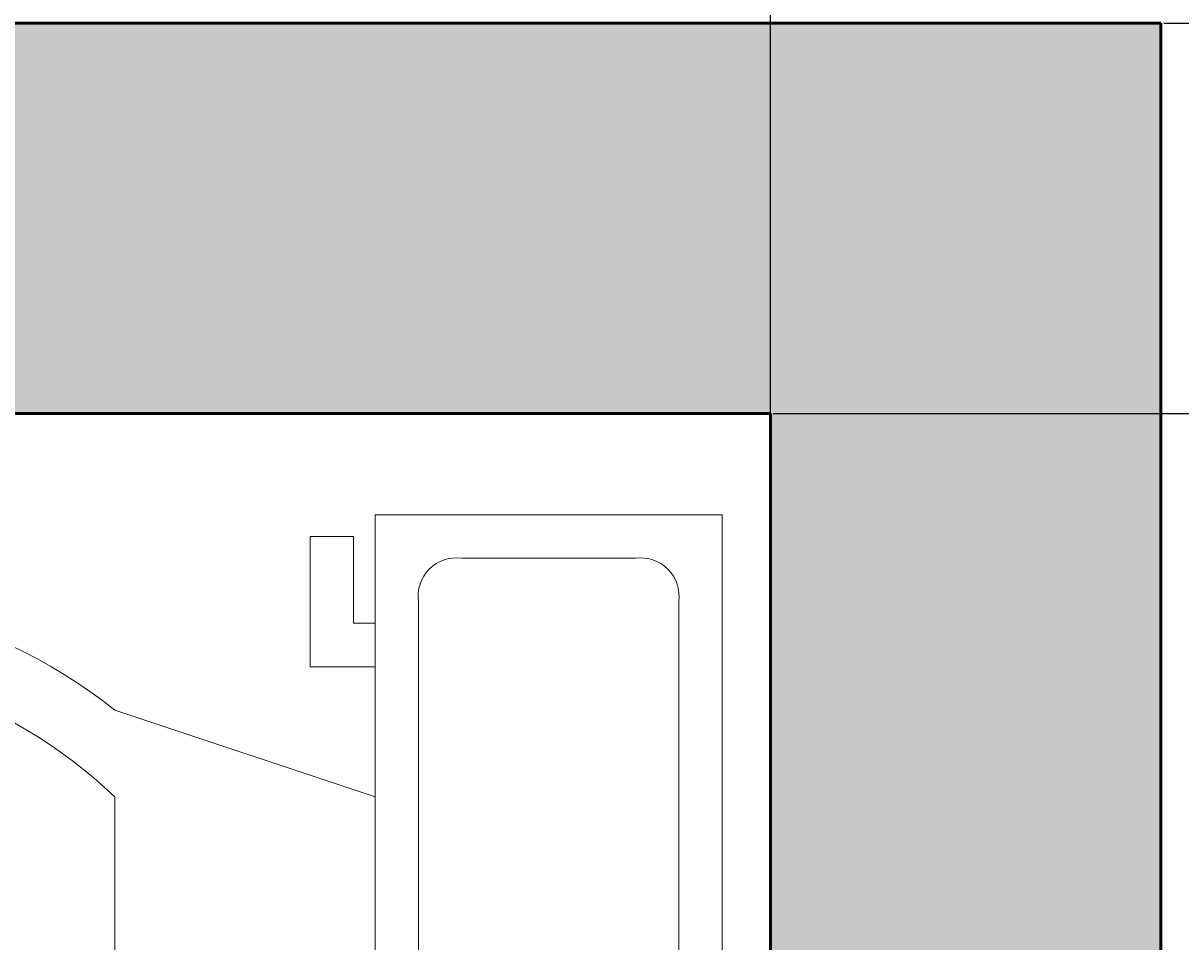
# Model space of a CAD drawing. Units: inches. Extents: x 2307 to 2544, y 2171 to 2540.
# Tile 50 of 52: x 2498 to 2525, y 2499 to 2521. Entities that reach past the tile are written whole.
import ezdxf

# ---------------------------------------------------------------- set-up
doc = ezdxf.new("R2010")
doc.units = ezdxf.units.IN
for name, color, linetype, lineweight in [('A-ANNO-DIMS', 2, 'Continuous', 18), ('A-FLOR-FIXT', 9, 'Continuous', 18), ('A-WALL', 7, 'Continuous', 50)]:
    doc.layers.add(name, color=color, linetype=linetype, lineweight=lineweight)
doc.layers.add('A-WALL-PATT', color=18, linetype='Continuous', lineweight=13, true_color=0x000000)
doc.styles.get("Standard").update_dxf_attribs({"font": 'arial.ttf'})
doc.dimstyles.get("Standard").update_dxf_attribs({"dimtxt": 0.18, "dimasz": 0.18, "dimexe": 0.18, "dimexo": 0.0625, "dimgap": 0.09, "dimtad": 0, "dimtih": 1, "dimtoh": 1, "dimdec": 4, "dimzin": 0, "dimdsep": 46, "dimtxsty": 'Standard', "dimcen": 0.09, "dimadec": 0, "dimazin": 0, "dimtfac": 1, "dimtdec": 4, "dimtofl": 0, "dimtmove": 0, "dimatfit": 3, "dimfxl": 1, "dimtolj": 1, "dimtzin": 0, "dimarcsym": 0})

# ---------------------------------------------------------------- blocks, each defined once
blk = doc.blocks.new('Toilet - top')
for p, q in [((-8, -8.5), (-8, -8)), ((-7, -8), (-7, -9.5)), ((-4, -8), (-6, -14)), ((-10, -8.5), (-8, -8.5)), ((-10, -9.5), (-10, -8.5)), ((-7, -9.5), (-10, -9.5)), ((4, -14), (-4, -14))]:
    blk.add_line(p, q)
blk.add_lwpolyline([(10.5, -8), (10.5, 0), (-10.5, 0), (-10.5, -8)], close=True)
for points in [[(8.5, -1), (-8.5, -1)], [(-9.5, -2), (-9.5, -6)], [(-8.5, -7), (8.5, -7)]]:
    blk.add_lwpolyline(points)
for centre, radius, start, end in [((-8.625, -1.875), 0.884, 81.8699, 188.1301), ((-8.625, -6.125), 0.884, 171.8699, 278.1301), ((3.52, -21.58), 12.169, 141.4691, 247.9714), ((4.2, -21.817), 11.329, 136.3677, 238.9468)]:
    blk.add_arc(centre, radius, start, end)
blk = doc.blocks.new('*D37')
at = {"layer": 'A-ANNO-DIMS', "color": 0, "lineweight": -2, "transparency": 16777216}
for p, q in [((2524.758, 2520.51), (2544.026, 2520.51)), ((2543.846, 2520.33), (2543.846, 2355.692)), ((2543.846, 2190.69), (2543.846, 2355.328)), ((2524.758, 2190.51), (2544.026, 2190.51))]:
    blk.add_line(p, q, dxfattribs=at)
at = {"layer": 'A-ANNO-DIMS', "color": 0, "transparency": 16777216}
for points in [[(2543.816, 2520.33), (2543.876, 2520.33), (2543.846, 2520.51)], [(2543.816, 2190.69), (2543.876, 2190.69), (2543.846, 2190.51)]]:
    blk.add_solid(points, dxfattribs=at)
at = {"layer": 'Defpoints', "color": 0, "transparency": 16777216}
for p in [(2524.696, 2520.51), (2543.846, 2520.51), (2524.696, 2190.51)]:
    blk.add_point(p, dxfattribs=at)
at = {"layer": 'A-ANNO-DIMS', "color": 0, "transparency": 16777216, "insert": (2543.846, 2355.51), "char_height": 0.18, "attachment_point": 5}
blk.add_mtext('\\A1;330', dxfattribs=at)
blk = doc.blocks.new('*D46')
at = {"layer": 'A-ANNO-DIMS', "color": 0, "lineweight": -2, "transparency": 16777216}
for p, q in [((2455.696, 2511.572), (2455.696, 2540.345)), ((2515.696, 2511.572), (2515.696, 2540.345)), ((2455.876, 2540.165), (2485.477, 2540.165)), ((2515.516, 2540.165), (2485.915, 2540.165))]:
    blk.add_line(p, q, dxfattribs=at)
at = {"layer": 'A-ANNO-DIMS', "color": 0, "transparency": 16777216}
for points in [[(2455.876, 2540.195), (2455.876, 2540.135), (2455.696, 2540.165)], [(2515.516, 2540.195), (2515.516, 2540.135), (2515.696, 2540.165)]]:
    blk.add_solid(points, dxfattribs=at)
at = {"layer": 'Defpoints', "color": 0, "transparency": 16777216}
for p in [(2515.696, 2540.165), (2455.696, 2511.51), (2515.696, 2511.51)]:
    blk.add_point(p, dxfattribs=at)
at = {"layer": 'A-ANNO-DIMS', "color": 0, "transparency": 16777216, "insert": (2485.696, 2540.165), "char_height": 0.18, "attachment_point": 5}
blk.add_mtext('\\A1;60', dxfattribs=at)
blk = doc.blocks.new('*D61')
at = {"layer": 'A-ANNO-DIMS', "color": 0, "lineweight": -2, "transparency": 16777216}
for p, q in [((2491.696, 2435.572), (2491.696, 2540.345)), ((2515.696, 2435.572), (2515.696, 2540.345)), ((2491.876, 2540.165), (2503.476, 2540.165)), ((2515.516, 2540.165), (2503.916, 2540.165))]:
    blk.add_line(p, q, dxfattribs=at)
at = {"layer": 'A-ANNO-DIMS', "color": 0, "transparency": 16777216}
for points in [[(2491.876, 2540.195), (2491.876, 2540.135), (2491.696, 2540.165)], [(2515.516, 2540.195), (2515.516, 2540.135), (2515.696, 2540.165)]]:
    blk.add_solid(points, dxfattribs=at)
at = {"layer": 'Defpoints', "color": 0, "transparency": 16777216}
for p in [(2515.696, 2540.165), (2491.696, 2435.51), (2515.696, 2435.51)]:
    blk.add_point(p, dxfattribs=at)
at = {"layer": 'A-ANNO-DIMS', "color": 0, "transparency": 16777216, "insert": (2503.696, 2540.165), "char_height": 0.18, "attachment_point": 5}
blk.add_mtext('\\A1;24', dxfattribs=at)
blk = doc.blocks.new('*D64')
at = {"layer": 'A-ANNO-DIMS', "color": 0, "lineweight": -2, "transparency": 16777216}
for p, q in [((2515.758, 2511.51), (2544.026, 2511.51)), ((2543.846, 2511.33), (2543.846, 2500.025)), ((2543.846, 2488.357), (2543.846, 2499.661)), ((2514.64, 2488.177), (2544.026, 2488.177))]:
    blk.add_line(p, q, dxfattribs=at)
at = {"layer": 'A-ANNO-DIMS', "color": 0, "transparency": 16777216}
for points in [[(2543.816, 2511.33), (2543.876, 2511.33), (2543.846, 2511.51)], [(2543.816, 2488.357), (2543.876, 2488.357), (2543.846, 2488.177)]]:
    blk.add_solid(points, dxfattribs=at)
at = {"layer": 'Defpoints', "color": 0, "transparency": 16777216}
for p in [(2515.696, 2511.51), (2514.578, 2488.177), (2543.846, 2488.177)]:
    blk.add_point(p, dxfattribs=at)
at = {"layer": 'A-ANNO-DIMS', "color": 0, "transparency": 16777216, "insert": (2543.846, 2499.843), "char_height": 0.18, "attachment_point": 5}
blk.add_mtext('\\A1;23.332', dxfattribs=at)

msp = doc.modelspace()

# ---------------------------------------------------------------- hatches: boundary and pattern name
at = {"layer": 'A-WALL-PATT'}
h = msp.add_hatch(color=256, dxfattribs=at)
h.dxf.hatch_style = 1
h.paths.add_polyline_path([(2433.6935, 2199.5096), (2415.6423, 2199.5096), (2415.6423, 2190.5096), (2433.7832, 2190.5096)], flags=17)
h.paths.add_polyline_path([(2367.6423, 2199.5096), (2335.6958, 2199.5096), (2335.6958, 2307.3983), (2326.6958, 2307.3983), (2326.6958, 2190.5096), (2367.6423, 2190.5096)])
h.paths.add_polyline_path([(2524.6958, 2520.5096), (2496.7832, 2520.5096), (2496.7832, 2515.5149), (2472.7832, 2515.5149), (2472.7832, 2520.5096), (2415.4028, 2520.5096), (2415.4028, 2511.5096), (2451.6958, 2511.5096), (2451.6958, 2439.5096), (2451.6958, 2391.5096), (2445.6958, 2391.5096), (2445.6958, 2387.5096), (2455.6958, 2387.5096), (2455.6958, 2435.5096), (2461.6958, 2435.5096), (2461.6958, 2439.5096), (2455.6958, 2439.5096), (2455.6958, 2511.5096), (2515.6958, 2511.5096), (2515.6958, 2439.5096), (2491.6958, 2439.5096), (2491.6958, 2435.5096), (2515.6958, 2435.5096), (2515.6958, 2319.5096), (2451.6958, 2319.5096), (2451.6958, 2281.5096), (2481.6958, 2281.5096), (2481.6958, 2225.5096), (2485.6958, 2225.5096), (2485.6958, 2285.5096), (2455.6958, 2285.5096), (2455.6958, 2315.5096), (2515.6958, 2315.5096), (2515.6958, 2199.5096), (2469.6952, 2199.5096), (2469.785, 2190.5096), (2524.6958, 2190.5096)])

# ---------------------------------------------------------------- linework, layer by layer
at = {"layer": 'A-WALL'}
for p, q in [((2455.6958, 2511.5096), (2515.6958, 2511.5096)), ((2515.6958, 2511.5096), (2515.6958, 2439.5096))]:
    msp.add_line(p, q, dxfattribs=at)
msp.add_lwpolyline([(2433.7832, 2190.5096), (2326.6958, 2190.5096), (2326.6958, 2520.5096), (2524.6958, 2520.5096), (2524.6958, 2190.5096), (2469.785, 2190.5096)], dxfattribs=at)

# ---------------------------------------------------------------- block references
at = {"layer": 'A-FLOR-FIXT', "rotation": 270}
msp.add_blockref('Toilet - top', (2514.5778, 2498.6772), dxfattribs=at)

# ---------------------------------------------------------------- dimensions: what is measured, and where the dimension line sits
at = {"layer": 'A-ANNO-DIMS'}
for p1, p2, picture, middle in [((2455.6958, 2511.5096), (2515.6958, 2511.5096), '*D46', (2485.6958, 2540.1649)), ((2491.6958, 2435.5096), (2515.6958, 2435.5096), '*D61', (2503.6958, 2540.1649))]:
    dim = msp.add_linear_dim(base=(2515.6958, 2540.1649), p1=p1, p2=p2, dimstyle='Standard', override={"dimdec": 0, "dimlfac": 1, "dimrnd": 0, "dimzin": 0, "dimdsep": 46, "dimlunit": 2}, dxfattribs=at)
    dim.commit()
    dim.dimension.update_dxf_attribs({"geometry": picture, "text_midpoint": middle})
for base, p1, p2, override, picture, middle in [((2543.8458, 2520.5096), (2524.6958, 2190.5096), (2524.6958, 2520.5096), {"dimdec": 0, "dimlfac": 1, "dimrnd": 0, "dimzin": 0, "dimdsep": 46, "dimlunit": 2}, '*D37', (2543.8458, 2355.5096)), ((2543.8458, 2488.1772), (2515.6958, 2511.5096), (2514.5778, 2488.1772), {"dimdec": 3, "dimlfac": 1, "dimrnd": 0, "dimzin": 0, "dimdsep": 46, "dimlunit": 2}, '*D64', (2543.8458, 2499.8434))]:
    dim = msp.add_linear_dim(base=base, p1=p1, p2=p2, angle=90, dimstyle='Standard', override=override, dxfattribs=at)
    dim.commit()
    dim.dimension.update_dxf_attribs({"geometry": picture, "text_midpoint": middle})

doc.saveas('drawing.dxf')
